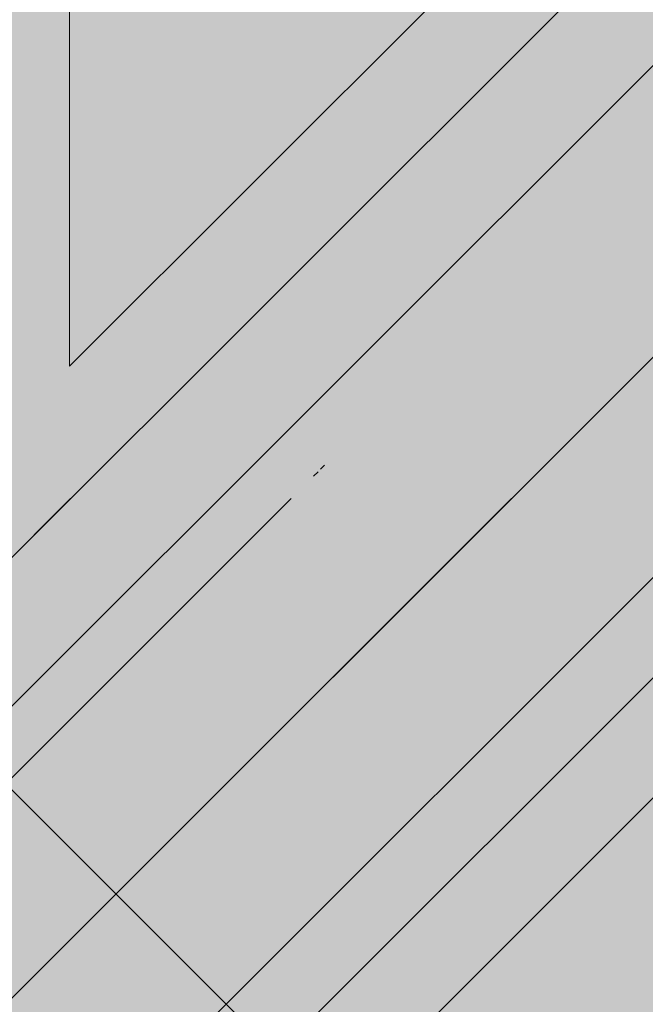
# Model space of a CAD drawing. Units: inches. Extents: x 844 to 2234, y 346 to 1084.
# Tile 11 of 93: x 1122.921 to 1123.72, y 691.183 to 692.442. Entities that reach past the tile are written whole.
import ezdxf

# ---------------------------------------------------------------- set-up
doc = ezdxf.new("R2010")
doc.units = ezdxf.units.IN
doc.header["$MEASUREMENT"] = 0
for name, color, linetype, lineweight in [('A-ANNO-DIMS', 2, 'Continuous', 18), ('furniture', 8, 'Continuous', 18), ('RA-AP-01$0$INT', 35, 'Continuous', 5)]:
    doc.layers.add(name, color=color, linetype=linetype, lineweight=lineweight)
doc.layers.add('RA-AP-01$0$FURN', color=3, linetype='Continuous')
doc.layers.add('RA-AP-01$0$WOOD', color=64, linetype='Continuous')
doc.styles.get("Standard").update_dxf_attribs({"font": 'arial.ttf'})
doc.dimstyles.get("Standard").update_dxf_attribs({"dimtxt": 6, "dimasz": 3, "dimexe": 0.18, "dimexo": 0.0625, "dimgap": 0.09, "dimtad": 0, "dimtih": 1, "dimtoh": 1, "dimdec": 1, "dimzin": 0, "dimdsep": 46, "dimlunit": 3, "dimtxsty": 'Standard', "dimblk": 'ARCHTICK', "dimcen": 0.09, "dimadec": 0, "dimazin": 0, "dimtfac": 1, "dimtdec": 1, "dimtofl": 0, "dimtmove": 0, "dimatfit": 3, "dimfxl": 1, "dimtolj": 1, "dimtzin": 0, "dimarcsym": 0})

# ---------------------------------------------------------------- blocks, each defined once
blk = doc.blocks.new('A$C18D01794')
at = {"layer": 'RA-AP-01$0$INT'}
h = blk.add_hatch(color=256, dxfattribs=at)
h.paths.add_polyline_path([(4.585917135068449, -6.356712009588271), (4.555206456959269, -6.35671200958746), (4.555206456959137, -6.387422687716308), (4.874495778835233, -6.706712009592356), (4.90520645695423, -6.676001331474049)])
h.paths.add_polyline_path([(5.255206456948813, -6.387422687716306), (5.255206456948682, -6.356712009605972), (5.224495778822613, -6.356712009605161), (4.905206456953498, -6.676001331474273), (4.935917135072151, -6.706712009592924)])
h.paths.add_polyline_path([(4.935917135072559, -6.706712009592068), (4.905206456953564, -6.737422687710376), (5.255206456951813, -7.087422687708613), (5.255206456951549, -7.026001331471008)])
h.paths.add_polyline_path([(4.555206456956399, -7.026001331471013), (4.555206456956134, -7.087422687708616), (4.905206456953821, -6.737422687710943), (4.874495778835166, -6.70671200959229)])
h = blk.add_hatch(color=256, dxfattribs=at)
h.paths.add_polyline_path([(4.585917135068448, -6.356712009588273), (4.614201406330596, -6.356712009589021), (4.668846067270487, -6.411356670531338), (4.723490728212344, -6.356712009591912), (4.771774999457151, -6.35671200959319), (4.826419660396886, -6.411356670535356), (4.862780050090322, -6.374996280843536), (4.844495778842715, -6.356712009595112), (4.862780050090411, -6.356712009595595), (4.905206456960182, -6.399138416468211), (4.947632863832445, -6.356712009597838), (4.965917135079675, -6.356712009598322), (4.947632863831759, -6.374996280845421), (4.983993253523576, -6.411356670538857), (5.038637914464627, -6.356712009600247), (5.08692218571208, -6.356712009601523), (5.141566846649976, -6.411356670541852), (5.196211507589851, -6.356712009604411), (5.224495778822615, -6.356712009605161), (4.905206456953975, -6.676001331473793)])
h.paths.add_polyline_path([(4.895206456956031, -6.637717060225675), (4.895206456958921, -6.528427738347902), (4.840561796018589, -6.583072399285802)], flags=16)
h.paths.add_polyline_path([(4.915206456955638, -6.637717060226121), (4.969851117895509, -6.583072399288678), (4.915206456957609, -6.528427738348344)], flags=16)
h.paths.add_polyline_path([(4.826419660395175, -6.568930263661755), (4.881064321335613, -6.514285602723745), (4.771774999456703, -6.514285602720857)], flags=16)
h.paths.add_polyline_path([(4.983993253519558, -6.568930263665262), (5.038637914460456, -6.514285602726792), (4.929348592581548, -6.514285602724816)], flags=16)
h.paths.add_polyline_path([(4.881064321336025, -6.494285602723742), (4.826419660397532, -6.439640941782821), (4.771774999457062, -6.494285602720859)], flags=16)
h.paths.add_polyline_path([(4.929348592582019, -6.494285602724817), (5.038637914460982, -6.494285602726792), (4.983993253522945, -6.439640941786327)], flags=16)
h.paths.add_polyline_path([(4.895206456960191, -6.480143467100443), (4.895206456962115, -6.407422687715913), (4.876922185715016, -6.389138416467584), (4.840561796021581, -6.425498806159401)], flags=16)
h.paths.add_polyline_path([(4.915206456958487, -6.480143467100889), (4.969851117899527, -6.425498806162279), (4.933490728206909, -6.389138416468043), (4.9152064569598, -6.40742268771434)], flags=16)
h.paths.add_polyline_path([(4.757632863832376, -6.480143467096812), (4.812277524772842, -6.425498806158772), (4.757632863834348, -6.370854145217844)], flags=16)
h.paths.add_polyline_path([(4.737632863832376, -6.480143467096286), (4.737632863834348, -6.370854145217375), (4.682988202893906, -6.425498806155385)], flags=16)
h.paths.add_polyline_path([(5.05278005008503, -6.480143467103376), (5.052780050087917, -6.370854145224413), (4.998135389146995, -6.425498806162908)], flags=16)
h.paths.add_polyline_path([(5.072780050085024, -6.480143467103744), (5.127424711025931, -6.42549880616527), (5.072780050087916, -6.370854145224832)], flags=16)
h.paths.add_polyline_path([(4.935917135072783, -6.706712009592292), (5.255206456948811, -6.387422687716309), (5.255206456948932, -6.415706958964177), (5.200561796010279, -6.470351619902839), (5.255206456949403, -6.524996280841948), (5.25520645694961, -6.5732805520894), (5.200561796009787, -6.627925213029239), (5.236922185702417, -6.664285602721864), (5.255206456949919, -6.646001331474357), (5.255206456949998, -6.664285602721898), (5.212780050078687, -6.706712009592262), (5.25520645695036, -6.749138416463932), (5.255206456950438, -6.767422687711313), (5.236922185702424, -6.749138416463297), (5.200561796009796, -6.785498806155928), (5.255206456950753, -6.840143467096874), (5.25520645695096, -6.888427738341682), (5.200561796010322, -6.943072399282328), (5.255206456951428, -6.997717060223427), (5.255206456951547, -7.026001331471006)])
h.paths.add_polyline_path([(5.042988202883395, -6.785498806155427), (5.097632863823085, -6.840143467095101), (5.097632863822622, -6.730854145216193)], flags=16)
h.paths.add_polyline_path([(5.028846067259663, -6.771356670531693), (5.083490728198774, -6.716712009592573), (4.974201406321001, -6.716712009593042)], flags=16)
h.paths.add_polyline_path([(5.117632863823087, -6.840143467095186), (5.172277524762331, -6.785498806155926), (5.11763286382262, -6.730854145216225)], flags=16)
h.paths.add_polyline_path([(5.08349072819877, -6.696712009593886), (5.028846067259652, -6.642067348654775), (4.974201406320998, -6.696712009593438)], flags=16)
h.paths.add_polyline_path([(5.131774999446817, -6.854285602718917), (5.186419660386065, -6.799640941779662), (5.241064321325782, -6.854285602719365)], flags=17)
h.paths.add_polyline_path([(5.131774999446228, -6.716712009592374), (5.186419660386065, -6.771356670532194), (5.222780050079488, -6.734996280838764), (5.204495778832781, -6.716712009592063)], flags=16)
h.paths.add_polyline_path([(5.097632863822613, -6.682569873970264), (5.097632863823061, -6.573280552091354), (5.042988202883383, -6.627925213031044)], flags=16)
h.paths.add_polyline_path([(5.131774999446899, -6.874285602718915), (5.241064321325809, -6.874285602719364), (5.186419660386591, -6.928930263658598)], flags=17)
h.paths.add_polyline_path([(5.131774999446226, -6.696712009594078), (5.204495778830767, -6.696712009594374), (5.22278005007868, -6.67842773834687), (5.186419660386049, -6.642067348654249)], flags=16)
h.paths.add_polyline_path([(5.11763286382262, -6.682569873970225), (5.17227752476232, -6.627925213030515), (5.117632863823064, -6.573280552091267)], flags=16)
h.paths.add_polyline_path([(5.186419660386069, -6.613783077405491), (5.241064321325754, -6.559138416465795), (5.131774999446791, -6.559138416466263)], flags=16)
h.paths.add_polyline_path([(5.131774999446872, -6.539138416466263), (5.24106432132578, -6.539138416465794), (5.186419660386554, -6.484493755526573)], flags=16)
h.paths.add_polyline_path([(5.255206456951811, -7.08742268770861), (5.255206456951895, -7.106712009588038), (4.555206456956052, -7.106712009588038), (4.555206456956136, -7.087422687708617), (4.905206456953973, -6.737422687710788)])
h.paths.add_polyline_path([(4.983993253513404, -6.8444937555241), (4.92934859257295, -6.899138416462108), (5.03863791445186, -6.899138416465014)], flags=16)
h.paths.add_polyline_path([(4.969851117889988, -6.83035161990006), (4.915206456952556, -6.775706958960171), (4.915206456949648, -6.884996280837944)], flags=16)
h.paths.add_polyline_path([(4.929348592572535, -6.919138416462105), (4.983993253511019, -6.973783077403037), (5.038637914451496, -6.919138416465012)], flags=16)
h.paths.add_polyline_path([(5.052780050074912, -6.93328055208906), (4.998135389134438, -6.987925213027088), (5.052780050072919, -7.042569873968025)], flags=16)
h.paths.add_polyline_path([(5.07278005007491, -6.933280552089588), (5.072780050072918, -7.042569873968497), (5.127424711013374, -6.987925213030498)], flags=16)
h.paths.add_polyline_path([(4.89520645695295, -6.775706958959721), (4.840561796013067, -6.830351619897157), (4.895206456950961, -6.884996280837494)], flags=16)
h.paths.add_polyline_path([(4.915206456948365, -6.933280552085403), (4.915206456946434, -7.006001331471951), (4.933490728192729, -7.024285602719066), (4.969851117886972, -6.987925213026453)], flags=16)
h.paths.add_polyline_path([(4.881064321327021, -6.899138416461022), (4.82641966038902, -6.84449375552057), (4.771774999448108, -6.899138416459029)], flags=16)
h.paths.add_polyline_path([(4.895206456950073, -6.933280552084951), (4.840561796009022, -6.987925213023558), (4.876922185700835, -7.024285602716997), (4.895206456948749, -7.006001331469487)], flags=16)
h.paths.add_polyline_path([(4.983993253510392, -7.0020673486505), (4.947632863816944, -7.038427738342319), (4.965917135064043, -7.05671200959023), (5.038637914448995, -7.056712009591555)], flags=16)
h.paths.add_polyline_path([(4.881064321326543, -6.91913841646102), (4.771774999447578, -6.919138416459031), (4.826419660385607, -6.973783077399508)], flags=16)
h.paths.add_polyline_path([(4.905206456946447, -7.014285602717636), (4.862780050074785, -7.056712009588352), (4.947632863816685, -7.056712009589775)], flags=16)
h.paths.add_polyline_path([(5.14156684663679, -7.002067348654549), (5.086922185696452, -7.056712009592438), (5.196211507574223, -7.056712009594425)], flags=16)
h.paths.add_polyline_path([(4.8264196603837, -7.002067348646972), (4.771774999442643, -7.056712009585575), (4.8444957788276, -7.056712009587508), (4.862780050075511, -7.038427738340416)], flags=16)
h.paths.add_polyline_path([(4.812277524760289, -6.98792521302292), (4.757632863822258, -6.933280552082447), (4.757632863819352, -7.042569873961408)], flags=16)
h.paths.add_polyline_path([(4.73763286382226, -6.933280552082079), (4.682988202881349, -6.987925213020536), (4.737632863819352, -7.04256987396099)], flags=16)
h.paths.add_polyline_path([(4.723490728195188, -7.056712009584289), (4.668846067257299, -7.002067348643949), (4.614201406317417, -7.056712009581383)], flags=16)
h.paths.add_polyline_path([(4.597632863829262, -6.706712009592262), (4.555206456957951, -6.664285602721896), (4.555206456958029, -6.646001331474357), (4.573490728205535, -6.664285602721864), (4.609851117898167, -6.627925213029238), (4.555206456958338, -6.573280552089402), (4.555206456958546, -6.524996280841952), (4.60985111789767, -6.470351619902839), (4.555206456959015, -6.415706958964177), (4.555206456959138, -6.387422687716309), (4.874495778835167, -6.70671200959229), (4.5552064569564, -7.026001331471015), (4.555206456956523, -6.997717060223433), (4.609851117897629, -6.94307239928233), (4.555206456956988, -6.888427738341681), (4.555206456957198, -6.840143467096881), (4.609851117898153, -6.78549880615593), (4.573490728205528, -6.749138416463297), (4.555206456957507, -6.76742268771132), (4.555206456957585, -6.749138416463933)])
h.paths.add_polyline_path([(4.712780050085332, -6.730854145216195), (4.712780050084863, -6.840143467095105), (4.767424711024555, -6.785498806155427)], flags=16)
h.paths.add_polyline_path([(4.726922185709173, -6.716712009592573), (4.781566846648288, -6.771356670531693), (4.836211507586949, -6.716712009593043)], flags=16)
h.paths.add_polyline_path([(4.692780050085327, -6.730854145216225), (4.638135389145619, -6.785498806155928), (4.692780050084865, -6.840143467095185)], flags=16)
h.paths.add_polyline_path([(4.726922185709182, -6.696712009593886), (4.836211507586949, -6.696712009593436), (4.7815668466483, -6.642067348654773)], flags=16)
h.paths.add_polyline_path([(4.678637914461726, -6.71671200959237), (4.605917135075169, -6.716712009592063), (4.587632863828464, -6.734996280838766), (4.623993253521887, -6.771356670532195)], flags=16)
h.paths.add_polyline_path([(4.712780050085336, -6.68256987397026), (4.767424711024568, -6.627925213031042), (4.71278005008489, -6.573280552091352)], flags=16)
h.paths.add_polyline_path([(4.678637914461726, -6.696712009594076), (4.623993253521899, -6.642067348654247), (4.587632863829271, -6.67842773834687), (4.605917135077185, -6.696712009594376)], flags=16)
h.paths.add_polyline_path([(4.692780050085336, -6.682569873970228), (4.692780050084889, -6.573280552091267), (4.638135389145632, -6.627925213030515)], flags=16)
h.paths.add_polyline_path([(4.623993253521885, -6.799640941779662), (4.678637914461131, -6.854285602718915), (4.56934859258217, -6.854285602719365)], flags=17)
h.paths.add_polyline_path([(4.623993253521901, -6.613783077405509), (4.678637914461158, -6.559138416466263), (4.569348592582195, -6.559138416465795)], flags=16)
h.paths.add_polyline_path([(4.678637914461051, -6.874285602718915), (4.623993253521361, -6.928930263658598), (4.569348592582143, -6.874285602719364)], flags=17)
h.paths.add_polyline_path([(4.678637914461076, -6.539138416466263), (4.623993253521399, -6.484493755526573), (4.569348592582167, -6.539138416465796)], flags=16)
h = blk.add_hatch(color=256, dxfattribs=at)
h.paths.add_polyline_path([(4.905206456953579, -6.70671200959253), (4.905206456953751, -6.676001331474523), (4.874495778835229, -6.706712009592358)])
h.paths.add_polyline_path([(4.935917135071924, -6.706712009592703), (4.905206456953583, -6.706712009592529), (4.90520645695341, -6.737422687710532)])
h = blk.add_hatch(color=256, dxfattribs=at)
h.paths.add_polyline_path([(4.895206456952951, -6.77570695895972), (4.840561796013068, -6.830351619897156), (4.895206456950958, -6.884996280837495)])
h.paths.add_polyline_path([(4.915206456949649, -6.884996280837942), (4.969851117889987, -6.830351619900054), (4.915206456952556, -6.775706958960171)])
h.paths.add_polyline_path([(5.038637914451862, -6.899138416465013), (4.983993253513403, -6.8444937555241), (4.929348592572953, -6.899138416462106)])
h.paths.add_polyline_path([(4.929348592572535, -6.919138416462105), (4.983993253511018, -6.973783077403037), (5.038637914451497, -6.919138416465012)])
h.paths.add_polyline_path([(4.915206456948366, -6.933280552085397), (4.915206456946433, -7.006001331471951), (4.93349072819273, -7.024285602719068), (4.969851117886972, -6.987925213026454)])
h.paths.add_polyline_path([(5.038637914448995, -7.056712009591553), (4.983993253510389, -7.002067348650502), (4.947632863816946, -7.038427738342318), (4.965917135064043, -7.05671200959023)])
h.paths.add_polyline_path([(5.05278005007292, -7.042569873968023), (5.05278005007491, -6.933280552089059), (4.998135389134438, -6.987925213027088)])
h.paths.add_polyline_path([(5.07278005007292, -7.042569873968496), (5.127424711013374, -6.987925213030498), (5.072780050074909, -6.933280552089588)])
h.paths.add_polyline_path([(5.141566846636789, -7.002067348654547), (5.086922185696449, -7.056712009592438), (5.196211507574223, -7.056712009594425)])
h.paths.add_polyline_path([(4.947632863816688, -7.056712009589774), (4.905206456946449, -7.014285602717634), (4.862780050074784, -7.056712009588353)])
h.paths.add_polyline_path([(4.840561796009025, -6.987925213023556), (4.876922185700834, -7.024285602716997), (4.895206456948747, -7.006001331469488), (4.895206456950075, -6.933280552084953)])
h.paths.add_polyline_path([(4.88106432132654, -6.919138416461021), (4.771774999447577, -6.919138416459031), (4.826419660385606, -6.973783077399508)])
h.paths.add_polyline_path([(4.881064321327019, -6.899138416461022), (4.826419660389019, -6.844493755520571), (4.771774999448108, -6.89913841645903)])
h.paths.add_polyline_path([(4.757632863819352, -7.042569873961409), (4.812277524760284, -6.987925213022922), (4.757632863822259, -6.933280552082447)])
h.paths.add_polyline_path([(4.8264196603837, -7.002067348646974), (4.771774999442646, -7.056712009585575), (4.844495778827599, -7.05671200958751), (4.862780050075512, -7.038427738340417)])
h.paths.add_polyline_path([(4.737632863819352, -7.042569873960988), (4.737632863822258, -6.933280552082078), (4.682988202881349, -6.987925213020538)])
h.paths.add_polyline_path([(4.668846067257299, -7.002067348643952), (4.61420140631742, -7.056712009581384), (4.723490728195189, -7.056712009584292)])
for p, q in [((4.935917135071927, -6.706712009592701), (4.905206456953407, -6.737422687710532)), ((4.935917135072783, -6.706712009592292), (5.255206456951548, -7.026001331471007)), ((4.905206456953975, -6.737422687710788), (5.255206456951811, -7.087422687708611)), ((4.915206456952556, -6.775706958960171), (4.969851117889986, -6.830351619900053)), ((4.915206456949648, -6.884996280837942), (4.915206456952556, -6.775706958960171))]:
    blk.add_line(p, q, dxfattribs=at)
blk = doc.blocks.new('A$C32926AE1')
at = {"layer": 'RA-AP-01$0$FURN'}
h = blk.add_hatch(dxfattribs=at)
h.set_pattern_fill('ANSI31', color=256, scale=0.1, style=0)
h.set_pattern_definition([(45, (0, 0), (-0.0088388347648318, 0.0088388347648318), [])])
edge = h.paths.add_edge_path(flags=16)
edge.add_arc((4.904771284329206, 4.246793130718756), 0.2603971832811541, 75.22398030683196, 104.7760196931204)
edge.add_arc((4.904771284329206, 4.246793130718756), 0.2603971832811541, 75.223980306832, 104.77601969312039, ccw=False)
edge = h.paths.add_edge_path(flags=16)
edge.add_arc((4.904771284329206, 4.067062675376612), 0.2603971832811541, 255.2239803068796, 284.776019693168)
edge.add_arc((4.904771284329206, 4.067062675376612), 0.2603971832811541, 255.22398030687958, 284.77601969316805, ccw=False)
edge = h.paths.add_edge_path(flags=0)
edge.add_arc((4.904771284329206, 4.067062675376612), 0.2603971832811541, 255.2239803068796, 284.776019693168)
edge.add_arc((4.904771284329206, 4.067062675376612), 0.2603971832811541, 255.22398030687958, 284.77601969316805, ccw=False)
edge = h.paths.add_edge_path(flags=0)
edge.add_arc((4.904771284329206, 4.067062675376612), 0.2603971832811541, 255.2239803068796, 284.776019693168)
edge.add_arc((4.904771284329206, 4.067062675376612), 0.2603971832811541, 255.22398030687958, 284.77601969316805, ccw=False)
edge = h.paths.add_edge_path()
edge.add_arc((4.604388392048174, 4.588829985554312), 0.1599999999999918, 342.3781640246255, 354.4317409793762)
edge.add_arc((5.090145208887507, 4.43216705527679), 0.3503971832811637, 162.0091218307731, 180.3186872093483)
edge.add_arc((5.205154176610243, 4.588829985554953), 0.1599999999999917, 185.5682590208461, 197.6218359767349)
edge.add_arc((4.904771284329229, 4.246793130718735), 0.3503971832811761, 72.00912183053516, 107.9908781690354)
edge.add_arc((9.535952835716557, 4.28682295566602), 4.798342501046485, 178.2875002453811, 181.5576802719453)
edge.add_arc((4.719397359771122, 4.43216705527679), 0.3503971832811637, 359.6813127906516, 377.9908781692269)
edge.add_arc((9.535967292294904, 4.286822350292874), 4.778371420254705, 178.2965938931842, 181.5667745797229)
edge.add_arc((4.719397359771122, 4.43216705527679), 0.3303971832811637, 359.6813127906516, 377.9908781692269)
edge.add_arc((0.2735752763637294, 4.286822350292874), 4.7783714202547, 358.4332254202771, 361.7034061068158)
edge.add_arc((5.061434214606998, 4.732549947558029), 0.1600000000000254, 252.3781640250584, 264.4317409792362)
edge.add_arc((4.748108354051257, 4.732549947558012), 0.1600000000000541, 275.5682590208426, 287.6218359759532)
edge.add_arc((4.604388392048115, 4.588829985554317), 0.1800000000000505, 342.3567572500182, 349.3735009646207)
edge.add_arc((5.205154176610254, 4.588829985554976), 0.1800000000000069, 190.6264990356027, 197.6432427513933)
edge.add_arc((5.061434214607106, 4.732549947558013), 0.1800000000000424, 252.3567572496606, 259.3735009644582)
edge.add_arc((4.904771284329208, 4.246793130718737), 0.3303971832811676, 71.99844483668534, 108.0015551637021)
edge.add_arc((4.748108354051414, 4.732549947558045), 0.1800000000000547, 280.6264990355479, 287.6432427495938)
edge.add_arc((5.090145208887514, 4.432167055276789), 0.2803971832811691, 162.8706300666893, 180.816523289902)
edge.add_arc((4.719397359771136, 4.432167055276689), 0.2803971832811534, 359.183476710103, 377.1293699333214)
edge.add_arc((4.904771284329222, 4.246793130718737), 0.2803971832811769, 72.87063006672916, 107.1293699332334)
edge.add_arc((5.090145208887522, 4.432167055276788), 0.2603971832811776, 165.2239803068007, 180.9953123810312)
edge.add_arc((4.719397359771141, 4.432167055276699), 0.2603971832811458, 359.0046876189768, 374.7760196932087)
edge.add_arc((5.090145208887507, 4.43216705527679), 0.3303971832811637, 162.0091218307731, 180.3186872093483)
edge.add_arc((9.53595427642584, 4.285015535491528), 4.728345371032053, 178.265043920078, 181.5679956281801)
edge.add_arc((0.2735882922327999, 4.285015535491582), 4.728345371032045, 358.4320043718193, 361.7349560799204)
edge.add_arc((9.535953591267507, 4.284458026472751), 4.708343996644348, 178.2573054306777, 181.5704995759608)
edge.add_arc((0.273588977391114, 4.284458026472785), 4.708343996644358, 358.4295004240388, 361.7426945693213)
edge.add_arc((0.2735889773911131, 4.029397779622582), 4.708343996644359, 358.2573054306787, 361.5704995759613)
edge.add_arc((9.535953591267518, 4.029397779622618), 4.708343996644359, 178.4295004240391, 181.7426945693223)
edge.add_arc((0.2735882922327901, 4.028840270603786), 4.728345371032054, 358.2650439200796, 361.5679956281808)
edge.add_arc((9.53595427642584, 4.028840270603841), 4.728345371032054, 178.4320043718199, 181.7349560799219)
edge.add_arc((0.2735752763637302, 4.027033455802493), 4.778371420254699, 358.2965938931842, 361.5667745797229)
edge.add_arc((4.719397359771122, 3.881688750818578), 0.3303971832811637, 342.0091218307731, 360.3186872093484)
edge.add_arc((5.090145208887507, 3.881688750818578), 0.3303971832811637, 179.6813127906516, 197.9908781692269)
edge.add_arc((9.535967292294904, 4.027033455802493), 4.778371420254705, 178.433225420277, 181.7034061068158)
edge.add_arc((4.719397359771122, 3.881688750818578), 0.3503971832811637, 342.0091218307731, 360.3186872093484)
edge.add_arc((9.53595283571655, 4.027032850429349), 4.79834250104648, 178.4423197280546, 181.7124997546188)
edge.add_arc((4.719397359771141, 3.881688750818669), 0.2603971832811458, 345.2239803067913, 360.9953123810232)
edge.add_arc((5.090145208887522, 3.88168875081858), 0.2603971832811776, 179.0046876189687, 194.7760196931993)
edge.add_arc((4.904771284329222, 4.067062675376631), 0.2803971832811769, 252.8706300667665, 287.1293699332708)
edge.add_arc((4.719397359771136, 3.881688750818678), 0.2803971832811534, 342.8706300666787, 360.8165232898969)
edge.add_arc((5.090145208887514, 3.881688750818579), 0.2803971832811691, 179.183476710098, 197.1293699333106)
edge.add_arc((4.748108354051414, 3.581305858537323), 0.1800000000000547, 72.3567572504062, 79.37350096445199)
edge.add_arc((4.904771284329208, 4.067062675376631), 0.3303971832811676, 251.9984448362979, 288.0015551633146)
edge.add_arc((5.061434214607106, 3.581305858537355), 0.1800000000000424, 100.6264990355418, 107.6432427503394)
edge.add_arc((5.205154176610254, 3.725025820540392), 0.1800000000000069, 162.3567572486066, 169.3735009643972)
edge.add_arc((4.604388392048115, 3.725025820541051), 0.1800000000000505, 10.62649903537925, 17.64324274998182)
edge.add_arc((4.748108354051257, 3.581305858537356), 0.1600000000000541, 72.37816402404681, 84.43174097915735)
edge.add_arc((4.904771284329229, 4.067062675376632), 0.3503971832811761, 252.0091218309645, 287.9908781694648)
edge.add_arc((5.061434214606998, 3.581305858537339), 0.1600000000000254, 95.56825902076373, 107.6218359749416)
edge.add_arc((5.205154176610243, 3.725025820540414), 0.1599999999999917, 162.3781640232651, 174.4317409791539)
edge.add_arc((5.090145208887507, 3.881688750818578), 0.3503971832811637, 179.6813127906516, 197.9908781692269)
edge.add_arc((4.604388392048174, 3.725025820541056), 0.1599999999999918, 5.568259020623824, 17.62183597537444)
edge.add_arc((0.2735897329420762, 4.28682295566602), 4.798342501046482, 358.4423197280547, 361.7124997546188)
edge.add_arc((0.2735897329420691, 4.027032850429348), 4.798342501046489, 358.2875002453812, 361.5576802719453)
at = {"layer": 'RA-AP-01$0$WOOD'}
h = blk.add_hatch(color=256, dxfattribs=at)
h.dxf.hatch_style = 1
h.paths.add_polyline_path([(5.157430609644524, 4.573483066760929, -0.1009492694046607), (5.155401577623758, 4.593365984175333, -0.1842662638101597), (5.172249623284174, 4.638795604568598, 0.2056608120311276), (5.179560981299304, 4.661316324430096, 0.3614336704623542), (5.134352340494423, 4.706524965234944, 0.2056608120311297), (5.111831620632933, 4.699213607219793, -0.1842662638101113), (5.066402000239693, 4.682365561559342, -0.1055311479399994), (5.045656153913092, 4.68467289944697, 0.1567636581983829), (4.763886414745334, 4.684672899446966, -0.1055311479399895), (4.743140568418733, 4.68236556155934, -0.1842662638100833), (4.6977109480255, 4.69921360721979, 0.2056608120302612), (4.675190228164109, 4.706524965234949, 0.3614336704708441), (4.629981587358889, 4.66131632442871, 0.2056608120245944), (4.637292945374126, 4.638795604567974, -0.1842662638101024), (4.654140991034615, 4.59336598417475, -0.1009492694055169), (4.652111959013835, 4.573483066760181, 0.021410119221476), (4.629748025606143, 4.156712009541676, 0.0214101192214795), (4.652111959013809, 3.739940952323101, -0.1009492694059586), (4.654140991034615, 3.720058034908448, -0.1842662638100975), (4.637292945374126, 3.674628414515226, 0.2056608120245705), (4.629981587358889, 3.652107694654492, 0.3614336704708879), (4.675190228164113, 3.606899053848249, 0.2056608120302384), (4.697710948025501, 3.614210411863408, -0.1842662638100995), (4.743140568418738, 3.63105845752386, -0.1055311479402541), (4.763886414745388, 3.628751119636215, 0.1567636581983776), (5.045656153913137, 3.628751119636244, -0.1055311479397538), (5.066402000239692, 3.631058457523857, -0.1842662638101067), (5.111831620632931, 3.614210411863407, 0.2056608120310924), (5.134352340494417, 3.606899053848256, 0.3614336704624001), (5.179560981299307, 3.652107694653103, 0.2056608120311314), (5.172249623284175, 3.6746284145146, -0.1842662638101402), (5.155401577623758, 3.72005803490786, -0.1009492694051366), (5.15743060964455, 3.739940952322354, 0.0214101192215073), (5.179794543052287, 4.156712009541468, 0.0214101192215252)])
h.paths.add_polyline_path([(4.639748609479751, 4.156712009541513, 0.0213537860821624), (4.661970494867118, 3.741887061152232, -0.094075836301374), (4.664143710413708, 3.7196126951003, -0.1824818158568985), (4.644813765429836, 3.668037719127816, 0.2056608120245319), (4.639939526753007, 3.653023905887301, 0.3614336704710246), (4.676106439397173, 3.616856993242342, 0.2056608120302234), (4.691120252638095, 3.621731231919122, -0.1824818158602558), (4.742695228611606, 3.641061176902986, -0.1029891339458722), (4.766991894714349, 3.638256818950944, 0.156709409989566), (5.042550673941472, 3.638256818950105, -0.102989133958497), (5.066847340047078, 3.641061176902949, -0.1824818158594995), (5.118422316020358, 3.621731231919103, 0.2056608120311416), (5.133436129261316, 3.616856993242346, 0.3614336704621468), (5.169603041905217, 3.653023905886178, 0.2056608120310986), (5.164728803228477, 3.668037719127177, -0.1824818158565612), (5.145398858244737, 3.719612695099578, -0.0940758363009313), (5.147572073791232, 3.741887061151398, 0.0213537860822023), (5.169793959178681, 4.156712009541451, 0.0213537860822226), (5.147572073791203, 4.571536957931898, -0.0940758363005034), (5.145398858244737, 4.59381132398362, -0.1824818158565587), (5.164728803228476, 4.645386299956021, 0.2056608120311045), (5.169603041905216, 4.66040011319702, 0.3614336704621845), (5.133436129261313, 4.696567025840856, 0.2056608120310773), (5.118422316020359, 4.691692787164098, -0.182481815859508), (5.066847340047078, 4.67236284218025, -0.1029891339584606), (5.04255067394148, 4.675167200133092, 0.156709409989566), (4.766991894714357, 4.675167200132257, -0.1029891339458842), (4.742695228611611, 4.672362842180213, -0.1824818158602725), (4.691120252638095, 4.691692787164077, 0.2056608120302152), (4.676106439397174, 4.696567025840858, 0.3614336704710363), (4.639939526753005, 4.660400113195899, 0.2056608120245495), (4.644813765429837, 4.645386299955384, -0.1824818158568934), (4.664143710413708, 4.593811323982902, -0.0940758363009187), (4.661970494867149, 4.571536957931074, 0.021353786082177)], flags=16)
h.paths.add_polyline_path([(5.129794543052235, 4.432167055276933, -0.0141661062790638), (5.130152669293814, 4.156927903047693, -0.0141661062790647), (5.129794543052234, 3.881688750818433, -0.0785247771143638), (5.10979738006795, 3.755143611847103, 0.0945969212073497), (5.105408519571111, 3.717898134952927, 0.1043170707844957), (5.116074640131521, 3.670385395016088, 0.1043170707864965), (5.068561900193738, 3.681051515576561, 0.09459692119553), (5.031316423304057, 3.676662655080835, -0.1580239521427272), (4.778226145355827, 3.676662655080367, 0.0945969211986668), (4.740980668464973, 3.681051515576592, 0.1043170707882822), (4.693467928526415, 3.670385395015844, 0.1043170707867916), (4.704134049087309, 3.717898134953662, 0.0945969211972894), (4.69974518859162, 3.755143611844042, -0.0785247771163196), (4.679748025606343, 3.881688750818406, -0.0141661062790663), (4.679389899364763, 4.156927903047693, -0.0141661062790672), (4.679748025606343, 4.432167055276998, -0.0785247771163064), (4.699745188591625, 4.55871219425134, 0.094596921197333), (4.704134049087308, 4.595957671141738, 0.1043170707867205), (4.693467928526416, 4.643470411079523, 0.1043170707882628), (4.740980668464965, 4.632804290518776, 0.0945969211988114), (4.778226145355874, 4.637193151015016, -0.158023952142669), (5.031316423304015, 4.637193151014546, 0.0945969211956361), (5.068561900193736, 4.632804290518806, 0.1043170707864979), (5.11607464013152, 4.643470411079278, 0.1043170707844617), (5.105408519571112, 4.595957671142455, 0.0945969212074597), (5.109797380067959, 4.558712194248236, -0.0785247771143467)], flags=0)
h.paths.add_polyline_path([(5.119794532311105, 4.432259799204851, -0.0142000800617244), (5.120156169157484, 4.156927903047701, -0.0142000800617277), (5.119794532311105, 3.881596006890482, -0.0784894509520253), (5.100273383573699, 3.758192358677797, 0.0940138827242913), (5.095413455884425, 3.717477693979438, 0.0606271852308753), (5.099615656341024, 3.686844378806616, 0.0606271852322524), (5.068982341167493, 3.691046579263239, 0.0940138827010453), (5.028267676478798, 3.686186651576848, -0.1580706864508061), (4.781274892180912, 3.686186651576435, 0.0940138827026903), (4.740560227491556, 3.691046579263279, 0.0606271852339895), (4.709926912317155, 3.686844378806508, 0.0606271852329405), (4.714129112773991, 3.717477693980356, 0.094013882701304), (4.709269185087677, 3.758192358669163, -0.0784894509577193), (4.689748036347473, 3.881596006890469, -0.014200080061729), (4.689386399501094, 4.156927903047709, -0.0142000800617217), (4.689748036347473, 4.432259799204808, -0.078489450957724), (4.709269185087651, 4.555663447426125, 0.0940138827014585), (4.714129112773992, 4.596378112114996, 0.0606271852329731), (4.709926912317154, 4.62701142728886, 0.0606271852340196), (4.74056022749157, 4.622809226832087, 0.0940138827024997), (4.781274892180847, 4.627669154518912, -0.1580706864508359), (5.028267676478777, 4.627669154518526, 0.0940138827010946), (5.068982341167492, 4.622809226832129, 0.060627185232254), (5.099615656341024, 4.627011427288751, 0.0606271852308727), (5.095413455884425, 4.59637811211593, 0.0940138827241088), (5.100273383573675, 4.555663447417647, -0.0784894509520978)], flags=0)
h.paths.add_polyline_path([(5.06978912287499, 4.430218106756144, -0.014241683694547), (5.070173729147532, 4.156927903047672, -0.0142416836945458), (5.06978912287499, 3.883637699339223, -0.0800609523125196), (5.052662118612511, 3.773463122773442, 0.0526421978001116), (5.04590916754064, 3.740550867606997, 0.0526421977992423), (5.012996912374707, 3.73379791653534, -0.1583028414718258), (4.796545656286308, 3.73379791653451, 0.0526421978034211), (4.763633401117837, 3.740550867607021, 0.0526421978018622), (4.756880450045755, 3.773463122774558, -0.0800609523117106), (4.739753445783639, 3.883637699339268, -0.0142416836945435), (4.739368839511098, 4.156927903047671, -0.0142416836945477), (4.739753445783639, 4.430218106756155, -0.0800609523116345), (4.75688045004574, 4.540392683320762, 0.052642197801941), (4.763633401117837, 4.573304938488346, 0.0526421978035071), (4.796545656286361, 4.580057889560873, -0.1583028414717561), (5.012996912374669, 4.580057889560039, 0.0526421977993048), (5.04590916754064, 4.57330493848837, 0.0526421978002057), (5.052662118612529, 4.540392683321868, -0.080060952312477)], flags=0)
h.paths.add_polyline_path([(5.049789715110557, 4.43038092723357, -0.0143097550741839), (5.05018085590259, 4.156927903047715, -0.0143097550741854), (5.049789715110558, 3.883474878861827, -0.0800685599149176), (5.03362098255317, 3.779581877367999, 0.0306258898956367), (5.028241146483733, 3.758218888663947, 0.0306258898977031), (5.006878157778253, 3.75283905259408, -0.1583983521624096), (4.802664410878162, 3.752839052594731, 0.0306258898946014), (4.781301422174808, 3.758218888663924, 0.0306258898967912), (4.775921586105202, 3.779581877368794, -0.080068559914251), (4.759752853548071, 3.883474878861786, -0.0143097550741854), (4.759361712756037, 4.156927903047671, -0.0143097550741854), (4.759752853548071, 4.430380927233557, -0.0800685599142479), (4.775921586105193, 4.534273928726546, 0.0306258898968306), (4.781301422174808, 4.555636917431444, 0.0306258898945754), (4.802664410878143, 4.561016753500631, -0.1583983521624168), (5.006878157778244, 4.561016753501291, 0.0306258898977177), (5.028241146483733, 4.555636917431421, 0.0306258898958182), (5.03362098255321, 4.534273928727244, -0.080068559914796)], flags=0)
h.paths.add_polyline_path([(4.999766070382627, 4.428171244713864, -0.0143443147609634), (5.000198441819402, 4.156927903047689, -0.0143443147609612), (4.999766070382627, 3.885684561381556, -0.0784641635803329), (4.987356730658798, 3.799103304488872, -0.1506053783831347), (4.822185837999821, 3.79910330448882, -0.0784641635803318), (4.809776498276007, 3.885684561381509, -0.014344314760963), (4.809344126839227, 4.156927903047677, -0.0143443147609645), (4.809776498276007, 4.428171244713873, -0.0784641635803192), (4.822185837999822, 4.514752501606549, -0.1506053783831338), (4.987356730658798, 4.514752501606494, -0.078464163580285)], flags=0)
h.paths.add_polyline_path([(4.979755254238824, 4.42764379880488, -0.0143772539198268), (4.980205517789977, 4.156927903047693, -0.0143772539198275), (4.979755254238824, 3.886212007290489, -0.0689242507424422), (4.971183264704897, 3.815276770442801, -0.1296645318904179), (4.838359303953726, 3.815276770442746, -0.0689242507424186), (4.829787314419809, 3.886212007290419, -0.0143772539198292), (4.829337050868653, 4.156927903047653, -0.0143772539198325), (4.829787314419809, 4.427643798804946, -0.0689242507424211), (4.838359303953725, 4.498579035652621, -0.1296645318904187), (4.971183264704897, 4.498579035652565, -0.0689242507424401)], flags=0)
h = blk.add_hatch(color=256, dxfattribs=at)
h.dxf.hatch_style = 1
h.paths.add_polyline_path([(5.145398858244737, 4.59381132398362, -0.1824818158565616), (5.164728803228476, 4.645386299956021, 0.2056608120311045), (5.169603041905216, 4.66040011319702, 0.3614336704621845), (5.133436129261313, 4.696567025840856, 0.2056608120310773), (5.118422316020359, 4.691692787164098, -0.182481815859508), (5.066847340047078, 4.67236284218025, -0.1029891339584606), (5.04255067394148, 4.675167200133092, 0.156709409989566), (4.766991894714357, 4.675167200132257, -0.1029891339458842), (4.742695228611611, 4.672362842180213, -0.1824818158602725), (4.691120252638095, 4.691692787164077, 0.2056608120302152), (4.676106439397174, 4.696567025840858, 0.3614336704710363), (4.639939526753005, 4.660400113195899, 0.2056608120245495), (4.644813765429837, 4.645386299955384, -0.1824818158568934), (4.664143710413708, 4.593811323982902, -0.0940758363009187), (4.661970494867149, 4.571536957931074, 0.0213537860821772), (4.639748609479751, 4.156712009541507, 0.0213537860821625), (4.661970494867119, 3.741887061152226, -0.0940758363013071), (4.664143710413708, 3.719612695100309, -0.1824818158569294), (4.644813765429836, 3.668037719127816, 0.2056608120245319), (4.639939526753007, 3.653023905887301, 0.3614336704710246), (4.676106439397173, 3.616856993242342, 0.2056608120302234), (4.691120252638095, 3.621731231919122, -0.1824818158602558), (4.742695228611606, 3.641061176902986, -0.1029891339458722), (4.766991894714349, 3.638256818950944, 0.156709409989566), (5.042550673941472, 3.638256818950105, -0.102989133958497), (5.066847340047078, 3.641061176902949, -0.1824818158594995), (5.118422316020358, 3.621731231919103, 0.2056608120311416), (5.133436129261316, 3.616856993242346, 0.3614336704621468), (5.169603041905217, 3.653023905886178, 0.2056608120310986), (5.164728803228477, 3.668037719127177, -0.1824818158565612), (5.145398858244737, 3.719612695099578, -0.0940758363009313), (5.147572073791232, 3.741887061151398, 0.0213537860822023), (5.169793959178681, 4.156712009541451, 0.0213537860822226), (5.147572073791203, 4.571536957931898, -0.0940758363004996)])
h.paths.add_polyline_path([(5.109797380067958, 4.55871219424824, -0.0785247771143472), (5.129794543052234, 4.432167055276936, -0.0141661062790644), (5.130152669293814, 4.156927903047685, -0.014166106279066), (5.129794543052234, 3.881688750818401, -0.0785247771143517), (5.109797380067946, 3.755143611847092, 0.0945969212073132), (5.105408519571111, 3.717898134952929, 0.1043170707844995), (5.116074640131521, 3.670385395016088, 0.1043170707864965), (5.068561900193738, 3.681051515576561, 0.09459692119553), (5.031316423304057, 3.676662655080835, -0.1580239521427272), (4.778226145355827, 3.676662655080367, 0.0945969211986668), (4.740980668464973, 3.681051515576592, 0.1043170707882822), (4.693467928526415, 3.670385395015844, 0.1043170707867916), (4.704134049087309, 3.717898134953662, 0.0945969211972894), (4.69974518859162, 3.755143611844042, -0.0785247771163196), (4.679748025606343, 3.881688750818406, -0.0141661062790663), (4.679389899364763, 4.156927903047693, -0.0141661062790672), (4.679748025606343, 4.432167055276998, -0.0785247771163064), (4.699745188591625, 4.55871219425134, 0.094596921197333), (4.704134049087308, 4.595957671141738, 0.1043170707867205), (4.693467928526416, 4.643470411079523, 0.1043170707882628), (4.740980668464965, 4.632804290518776, 0.0945969211988114), (4.778226145355874, 4.637193151015016, -0.158023952142669), (5.031316423304015, 4.637193151014546, 0.0945969211956361), (5.068561900193736, 4.632804290518806, 0.1043170707864979), (5.11607464013152, 4.643470411079278, 0.1043170707844617), (5.105408519571112, 4.595957671142455, 0.0945969212074504)], flags=16)
h.paths.add_polyline_path([(5.100273383573655, 4.55566344741771, -0.0784894509521388), (5.119794532311105, 4.432259799204852, -0.0142000800617252), (5.120156169157484, 4.156927903047686, -0.014200080061726), (5.119794532311105, 3.881596006890502, -0.0784894509520446), (5.100273383573696, 3.758192358677786, 0.0940138827242721), (5.095413455884425, 3.717477693979436, 0.0606271852308692), (5.099615656341024, 3.686844378806616, 0.0606271852322522), (5.068982341167493, 3.691046579263239, 0.0940138827010453), (5.028267676478798, 3.686186651576848, -0.1580706864508061), (4.781274892180912, 3.686186651576435, 0.0940138827026903), (4.740560227491556, 3.691046579263279, 0.0606271852339895), (4.709926912317155, 3.686844378806508, 0.0606271852329405), (4.714129112773991, 3.717477693980356, 0.094013882701304), (4.709269185087677, 3.758192358669163, -0.0784894509577193), (4.689748036347473, 3.881596006890469, -0.014200080061729), (4.689386399501094, 4.156927903047709, -0.0142000800617217), (4.689748036347473, 4.432259799204808, -0.078489450957724), (4.709269185087651, 4.555663447426125, 0.0940138827014585), (4.714129112773992, 4.596378112114996, 0.0606271852329731), (4.709926912317154, 4.62701142728886, 0.0606271852340196), (4.74056022749157, 4.622809226832087, 0.0940138827024997), (4.781274892180847, 4.627669154518912, -0.1580706864508359), (5.028267676478777, 4.627669154518526, 0.0940138827010946), (5.068982341167492, 4.622809226832129, 0.060627185232254), (5.099615656341024, 4.627011427288751, 0.0606271852308727), (5.095413455884425, 4.59637811211593, 0.094013882723957)], flags=0)
h.paths.add_polyline_path([(5.04590916754064, 4.57330493848837, 0.0526421978002057), (5.052662118612529, 4.540392683321868, -0.0800609523124783), (5.06978912287499, 4.430218106756142, -0.0142416836945469), (5.070173729147532, 4.156927903047672, -0.0142416836945458), (5.06978912287499, 3.883637699339223, -0.0800609523125196), (5.052662118612511, 3.773463122773442, 0.0526421978001116), (5.04590916754064, 3.740550867606997, 0.0526421977992423), (5.012996912374707, 3.73379791653534, -0.1583028414718258), (4.796545656286308, 3.73379791653451, 0.0526421978034211), (4.763633401117837, 3.740550867607021, 0.0526421978018622), (4.756880450045755, 3.773463122774558, -0.0800609523117106), (4.739753445783639, 3.883637699339268, -0.0142416836945435), (4.739368839511098, 4.156927903047671, -0.0142416836945477), (4.739753445783639, 4.430218106756155, -0.0800609523116345), (4.75688045004574, 4.540392683320762, 0.052642197801941), (4.763633401117837, 4.573304938488346, 0.0526421978035071), (4.796545656286361, 4.580057889560873, -0.1583028414717561), (5.012996912374669, 4.580057889560039, 0.0526421977993048)], flags=0)
h.paths.add_polyline_path([(5.028241146483733, 4.555636917431422, 0.0306258898956949), (5.033620982553182, 4.534273928727329, -0.0800685599148649), (5.049789715110557, 4.430380927233569, -0.0143097550741839), (5.05018085590259, 4.156927903047715, -0.0143097550741854), (5.049789715110558, 3.883474878861827, -0.0800685599149176), (5.03362098255317, 3.779581877367999, 0.0306258898956367), (5.028241146483733, 3.758218888663947, 0.0306258898977031), (5.006878157778253, 3.75283905259408, -0.1583983521624096), (4.802664410878162, 3.752839052594731, 0.0306258898946014), (4.781301422174808, 3.758218888663924, 0.0306258898967912), (4.775921586105202, 3.779581877368794, -0.080068559914251), (4.759752853548071, 3.883474878861786, -0.0143097550741854), (4.759361712756037, 4.156927903047671, -0.0143097550741854), (4.759752853548071, 4.430380927233557, -0.0800685599142479), (4.775921586105193, 4.534273928726546, 0.0306258898968306), (4.781301422174808, 4.555636917431444, 0.0306258898945754), (4.802664410878143, 4.561016753500631, -0.1583983521624168), (5.006878157778244, 4.561016753501291, 0.0306258898977174)], flags=0)
h.paths.add_polyline_path([(4.987356730658798, 4.514752501606494, -0.0784641635803018), (4.999766070382627, 4.428171244713845, -0.0143443147609637), (5.000198441819402, 4.156927903047665, -0.0143443147609622), (4.999766070382628, 3.885684561381514, -0.0784641635802952), (4.987356730658797, 3.799103304488872, -0.1506053783831338), (4.822185837999821, 3.799103304488819, -0.0784641635803342), (4.809776498276007, 3.885684561381512, -0.0143443147609628), (4.809344126839227, 4.156927903047676, -0.0143443147609646), (4.809776498276007, 4.428171244713873, -0.0784641635803192), (4.822185837999822, 4.514752501606549, -0.1506053783831338)], flags=0)
h.paths.add_polyline_path([(4.971183264704897, 4.498579035652566, -0.0689242507424384), (4.979755254238824, 4.427643798804883, -0.0143772539198276), (4.980205517789977, 4.15692790304768, -0.0143772539198258), (4.979755254238823, 3.88621200729051, -0.0689242507424628), (4.971183264704897, 3.815276770442801, -0.129664531890417), (4.838359303953726, 3.815276770442746, -0.0689242507424186), (4.829787314419809, 3.886212007290419, -0.0143772539198292), (4.829337050868653, 4.156927903047653, -0.0143772539198325), (4.829787314419809, 4.427643798804946, -0.0689242507424211), (4.838359303953725, 4.498579035652621, -0.1296645318904187)], flags=0)
h = blk.add_hatch(dxfattribs=at)
h.set_pattern_fill('ANSI31', color=256, scale=0.05, style=0)
h.set_pattern_definition([(45, (0, 0), (-0.0044194173824159, 0.0044194173824159), [])])
h.paths.add_polyline_path([(5.130152669293814, 4.156927903047704, 0.0141661062790657), (5.129794543052234, 4.432167055276982, 0.0777827904001433), (5.110168979996553, 4.557559993161921, -0.0976515123401879), (5.105408519571111, 4.595957671142454, -0.1043170707844687), (5.116074640131522, 4.64347041107928), (5.099615656341024, 4.627011427288751, 0.0606271852308727), (5.095413455884425, 4.59637811211593, 0.0940138827241088), (5.100273383573675, 4.555663447417647, -0.0784894509520972), (5.119794532311105, 4.432259799204852, -0.0142000800617252), (5.120156169157484, 4.156927903047686, -0.014200080061726), (5.119794532311105, 3.881596006890502, -0.0784894509520446), (5.100273383573696, 3.758192358677786, 0.0940138827242721), (5.095413455884425, 3.717477693979436, 0.0606271852308692), (5.099615656341024, 3.686844378806616), (5.116074640131519, 3.67038539501609, -0.1043170707844594), (5.105408519571112, 3.717898134952912, -0.0976515123401594), (5.11016897999655, 3.756295812933435, 0.0777827904001654), (5.129794543052234, 3.881688750818409, 0.0141661062790665)])
h.paths.add_polyline_path([(5.030164222210597, 3.676291055149937, -0.0976515123472002), (5.068561900193739, 3.681051515576561, -0.1043170707864927), (5.116074640131521, 3.670385395016088), (5.099615656341024, 3.686844378806616, 0.0606271852322522), (5.068982341167493, 3.691046579263239, 0.0940138827010453), (5.028267676478798, 3.686186651576848, -0.1580706864508061), (4.781274892180912, 3.686186651576435, 0.0940138827026903), (4.740560227491556, 3.691046579263279, 0.0606271852339913), (4.709926912317154, 3.686844378806508), (4.693467928526416, 3.670385395015845, -0.1043170707882796), (4.740980668464973, 3.681051515576592, -0.0976515123427246), (4.779378346446416, 3.676291055150394, 0.156512506893803)])
h.paths.add_polyline_path([(4.689748036347473, 3.881596006890472, -0.014200080061729), (4.689386399501094, 4.156927903047712, -0.0142000800617195), (4.689748036347473, 4.432259799204768, -0.078489450957742), (4.709269185087648, 4.555663447426114, 0.0940138827014821), (4.714129112773992, 4.596378112114995, 0.0606271852329748), (4.709926912317154, 4.62701142728886), (4.693467928526414, 4.643470411079524, -0.1043170707867939), (4.704134049087309, 4.595957671141706, -0.09765151234893), (4.699373588660725, 4.557559993157876, 0.0777827903975372), (4.679748025606343, 4.432167055276987, 0.0141661062790675), (4.679389899364763, 4.156927903047675, 0.0141661062790641), (4.679748025606343, 3.88168875081843, 0.0777827903975637), (4.699373588660724, 3.756295812937497, -0.0976515123490278), (4.704134049087308, 3.717898134953629, -0.1043170707867196), (4.693467928526416, 3.670385395015845), (4.709926912317155, 3.686844378806508, 0.0606271852329413), (4.714129112773991, 3.717477693980357, 0.0940138827013084), (4.709269185087676, 3.758192358669166, -0.0784894509577192)])
h.paths.add_polyline_path([(4.779378346446434, 4.63756475094498, -0.0976515123427943), (4.740980668464964, 4.632804290518776, -0.1043170707882609), (4.693467928526416, 4.643470411079523), (4.709926912317154, 4.62701142728886, 0.0606271852340196), (4.74056022749157, 4.622809226832087, 0.0940138827024997), (4.781274892180847, 4.627669154518912, -0.1580706864508359), (5.028267676478777, 4.627669154518526, 0.0940138827010946), (5.068982341167492, 4.622809226832129, 0.060627185232254), (5.099615656341024, 4.627011427288751), (5.116074640131521, 4.643470411079279, -0.1043170707865022), (5.068561900193735, 4.632804290518806, -0.0976515123475899), (5.030164222210446, 4.637564750945479, 0.1565125068936924)])
h = blk.add_hatch(dxfattribs=at)
h.set_pattern_fill('ANSI32', color=256, scale=0.2, style=0)
h.set_pattern_definition([(45, (0, 0), (-0.0530330085889911, 0.0530330085889911), []), (45, (0.035355339, 0), (-0.0530330085889911, 0.0530330085889911), [])])
h.paths.add_polyline_path([(5.119794532311105, 4.432259799204823, 0.0777015974868765), (5.10065834347252, 4.554469821747928, -0.0968902511992216), (5.095413455884425, 4.596378112115931, -0.060627185230871), (5.099615656341024, 4.627011427288751, -0.060627185232254), (5.068982341167492, 4.622809226832129, -0.0968902512198245), (5.027074050790956, 4.628054114423209, 0.1564657949319105), (4.782468517866163, 4.628054114422785, -0.0968902512152247), (4.740560227491555, 4.622809226832088, -0.0606271852339878), (4.709926912317155, 4.627011427288859, -0.0606271852329413), (4.714129112773991, 4.596378112115011, -0.0968902512205338), (4.708884225182929, 4.554469821738175, 0.0777015974804443), (4.689748036347473, 4.43225979920482, 0.0142000800617215), (4.689386399501094, 4.156927903047726, 0.0142000800617273), (4.689748036347473, 3.88159600689052, 0.077701597480541), (4.708884225182985, 3.759385984357019, -0.096890251220082), (4.714129112773992, 3.717477693980371, -0.0606271852329731), (4.709926912317154, 3.686844378806507, -0.060627185233988), (4.740560227491554, 3.691046579263279, -0.0968902512152569), (4.782468517866175, 3.685801691672578, 0.1564657949319236), (5.027074050790988, 3.685801691672169, -0.0968902512197451), (5.068982341167491, 3.691046579263239, -0.0606271852322557), (5.099615656341024, 3.686844378806616, -0.0606271852308727), (5.095413455884425, 3.717477693979438, -0.0968902511991229), (5.100658343472507, 3.7593859843474, 0.0777015974868745), (5.119794532311105, 3.8815960068905, 0.014200080061726), (5.120156169157484, 4.156927903047685, 0.0142000800617238)])
h.paths.add_polyline_path([(5.070173729147531, 4.156927903047684, -0.0142416836945481), (5.06978912287499, 3.883637699339191, -0.0800609523125107), (5.052662118612505, 3.773463122773424, 0.0526421978000811), (5.04590916754064, 3.740550867606997, 0.0526421977993214), (5.012996912374658, 3.733797916535325, -0.1583028414717916), (4.796545656286304, 3.733797916534512, 0.0526421978034138), (4.763633401117837, 3.740550867607021, 0.0526421978018622), (4.756880450045755, 3.773463122774558, -0.0800609523117106), (4.739753445783639, 3.883637699339268, -0.0142416836945435), (4.739368839511098, 4.156927903047671, -0.0142416836945477), (4.739753445783639, 4.430218106756155, -0.0800609523116345), (4.75688045004574, 4.540392683320762, 0.052642197801941), (4.763633401117837, 4.573304938488346, 0.0526421978035071), (4.796545656286361, 4.580057889560873, -0.1583028414717561), (5.012996912374669, 4.580057889560039, 0.0526421977993048), (5.04590916754064, 4.57330493848837, 0.0526421978002057), (5.052662118612529, 4.540392683321868, -0.0800609523124783), (5.06978912287499, 4.430218106756142, -0.0142416836945463)], flags=16)
h.paths.add_polyline_path([(5.050180855902591, 4.156927903047686, -0.0143097550741856), (5.049789715110558, 3.883474878861795, -0.0800685599148126), (5.033620982553202, 3.7795818773681, 0.0306258898957837), (5.028241146483733, 3.758218888663947, 0.0306258898977031), (5.006878157778253, 3.75283905259408, -0.1583983521624096), (4.802664410878162, 3.752839052594731, 0.0306258898946014), (4.781301422174808, 3.758218888663924, 0.0306258898967912), (4.775921586105202, 3.779581877368794, -0.080068559914251), (4.759752853548071, 3.883474878861786, -0.0143097550741854), (4.759361712756037, 4.156927903047671, -0.0143097550741854), (4.759752853548071, 4.430380927233557, -0.0800685599142479), (4.775921586105193, 4.534273928726546, 0.0306258898968306), (4.781301422174808, 4.555636917431444, 0.0306258898945754), (4.802664410878143, 4.561016753500631, -0.1583983521624168), (5.006878157778244, 4.561016753501291, 0.0306258898977177), (5.028241146483733, 4.555636917431421, 0.0306258898958182), (5.03362098255321, 4.534273928727244, -0.0800685599147973), (5.049789715110557, 4.430380927233568, -0.0143097550741854)], flags=0)
h.paths.add_polyline_path([(5.000198441819402, 4.15692790304769, -0.0143443147609622), (4.999766070382627, 3.885684561381539, -0.0784641635803169), (4.987356730658798, 3.799103304488873, -0.1506053783831347), (4.822185837999821, 3.79910330448882, -0.0784641635803318), (4.809776498276007, 3.885684561381509, -0.014344314760963), (4.809344126839227, 4.156927903047677, -0.0143443147609645), (4.809776498276007, 4.428171244713873, -0.0784641635803192), (4.822185837999822, 4.514752501606549, -0.1506053783831338), (4.987356730658798, 4.514752501606494, -0.0784641635803018), (4.999766070382627, 4.428171244713845, -0.0143443147609624)], flags=0)
h.paths.add_polyline_path([(4.980205517789976, 4.156927903047707, -0.0143772539198295), (4.979755254238824, 3.886212007290466, -0.06892425074242), (4.971183264704897, 3.815276770442801, -0.129664531890417), (4.838359303953726, 3.815276770442746, -0.0689242507424186), (4.829787314419809, 3.886212007290419, -0.0143772539198292), (4.829337050868653, 4.156927903047653, -0.0143772539198325), (4.829787314419809, 4.427643798804946, -0.0689242507424211), (4.838359303953725, 4.498579035652621, -0.1296645318904187), (4.971183264704897, 4.498579035652565, -0.0689242507424418), (4.979755254238824, 4.427643798804878, -0.0143772539198259)], flags=0)
blk = doc.blocks.new('A$C5D2F253E')
at = {"layer": 'RA-AP-01$0$FURN', "xscale": -0.7999999999883585, "yscale": 0.7999999999883585, "zscale": 0.8, "rotation": 90}
blk.add_blockref('A$C18D01794', (-5.687757199772477, 4.75791982714071), dxfattribs=at)
at = {"layer": 'RA-AP-01$0$WOOD', "rotation": 270}
blk.add_blockref('A$C32926AE1', (-4.161339601644158, 5.73852594588169), dxfattribs=at)
blk = doc.blocks.new('_ArchTick')
at = {"color": 0, "linetype": 'ByBlock', "const_width": 0.15}
blk.add_lwpolyline([(-0.5, -0.5), (0.5, 0.5)], dxfattribs=at)
blk = doc.blocks.new('*D144')
at = {"layer": 'A-ANNO-DIMS', "color": 0, "lineweight": -2, "transparency": 16777216}
for p, q in [((1096.615948, 439.3732739999999), (1096.615948, 1074.743301)), ((1143.115948, 492.373274), (1143.115948, 1074.743301)), ((1096.615948, 1074.563301), (1102.481950728513, 1074.563301)), ((1143.115948, 1074.563301), (1137.249945271487, 1074.563301))]:
    blk.add_line(p, q, dxfattribs=at)
at = {"layer": 'Defpoints', "color": 0, "transparency": 16777216}
for p in [(1143.115948, 1074.563301), (1143.115948, 492.3107739999999), (1096.615948, 439.3107739999999)]:
    blk.add_point(p, dxfattribs=at)
at = {"layer": 'A-ANNO-DIMS', "color": 0, "lineweight": -2, "transparency": 16777216, "xscale": 3, "yscale": 3, "zscale": 3, "rotation": 180}
blk.add_blockref('_ArchTick', (1096.615948, 1074.563301), dxfattribs=at)
at = {"layer": 'A-ANNO-DIMS', "color": 0, "lineweight": -2, "transparency": 16777216, "xscale": 3, "yscale": 3, "zscale": 3}
blk.add_blockref('_ArchTick', (1143.115948, 1074.563301), dxfattribs=at)
at = {"layer": 'A-ANNO-DIMS', "color": 0, "transparency": 16777216, "insert": (1119.865948, 1074.563301), "char_height": 6, "attachment_point": 5}
blk.add_mtext('\\A1;3\'-10 1/2"', dxfattribs=at)

msp = doc.modelspace()

# ---------------------------------------------------------------- block references
at = {"layer": 'furniture', "xscale": 15.94108302203742, "yscale": 15.94108302203742, "zscale": 15.94108302203742, "rotation": 90}
msp.add_blockref('A$C5D2F253E', (1136.147844094663, 696.2584716700112), dxfattribs=at)

# ---------------------------------------------------------------- dimensions: what is measured, and where the dimension line sits
at = {"layer": 'A-ANNO-DIMS'}
dim = msp.add_linear_dim(base=(1143.115948, 1074.563301), p1=(1096.615948, 439.3107739999999), p2=(1143.115948, 492.3107739999999), dimstyle='Standard', override={"dimdec": 1, "dimlfac": 1, "dimrnd": 0, "dimzin": 1, "dimdsep": 46, "dimlunit": 4, "dimfrac": 2}, dxfattribs=at)
dim.commit()
dim.dimension.update_dxf_attribs({"geometry": '*D144', "text_midpoint": (1119.865948, 1074.563301)})

doc.saveas('drawing.dxf')
